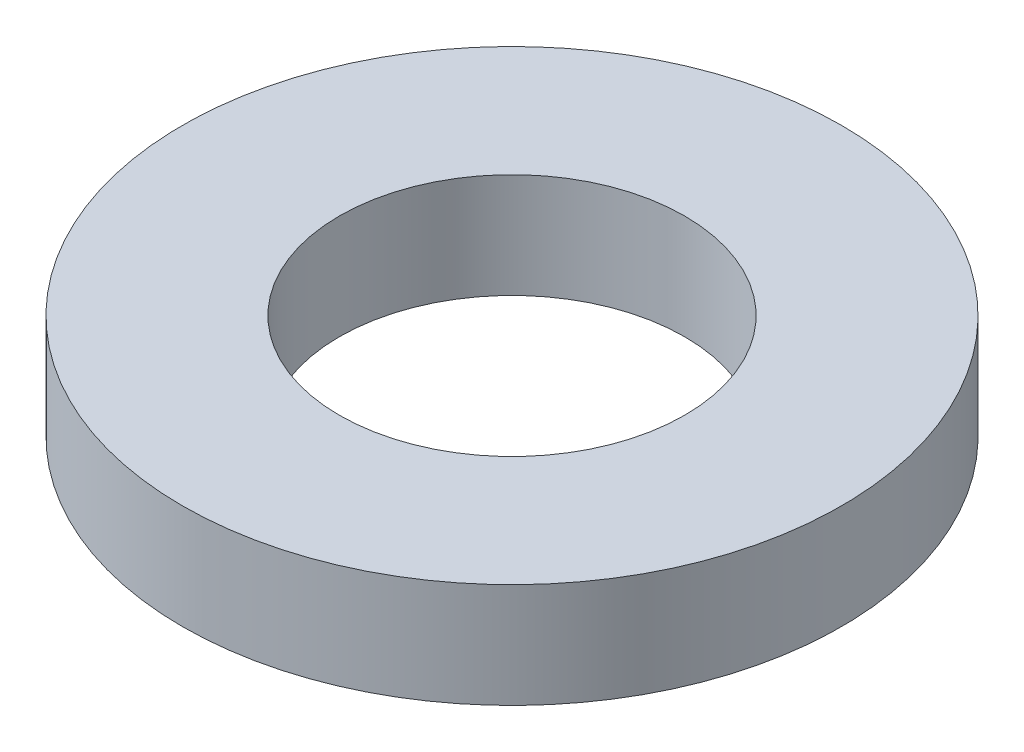
SolidWorks part; units mm, degrees
material "Plain Carbon Steel"
ref_plane "Front Plane" through (0, 0, 0) normal (0, 0, 1) x (1, 0, 0)
ref_plane "Top Plane" through (0, 0, 0) normal (0, 1, 0) x (1, 0, 0)
ref_plane "Right Plane" through (0, 0, 0) normal (1, 0, 0) x (0, 0, -1)
sketch "Washer Profile Ø63 x Ø33" plane through (0, 0, 0) normal (0, 1, 0) x (1, 0, 0)
  circle A0 centre (0, 0) radius 16.5
  circle A1 centre (0, 0) radius 31.5
  dimension "D1" = 33
  dimension "D2" = 63
extrude "Washer Body 10mm" add sketch "Washer Profile Ø63 x Ø33" along normal mid plane 10
